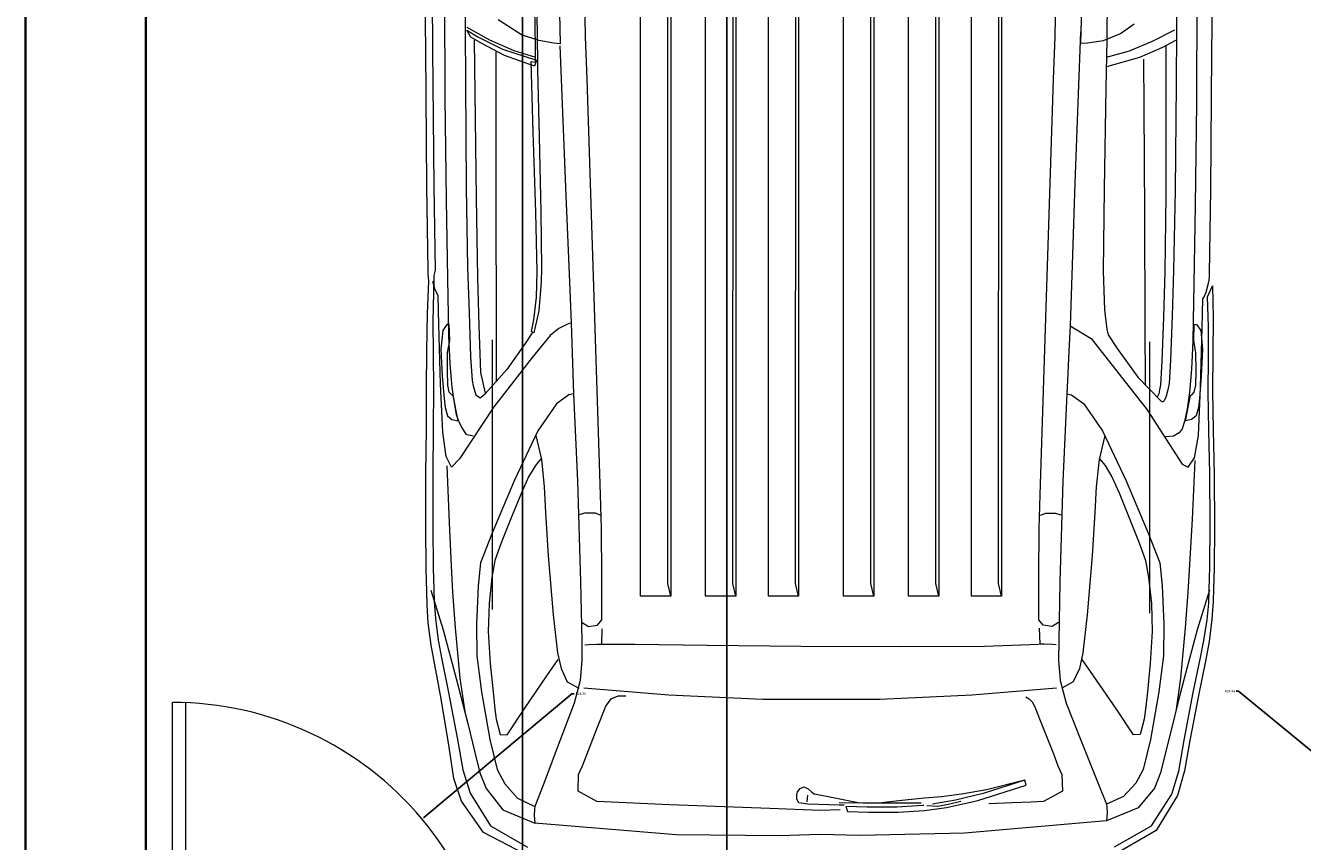
# Model space of a CAD drawing. Units: inches. Extents: x 5 to 421, y -617 to 43.
# Tile 2 of 15: x 37 to 133, y -566 to -505. Entities that reach past the tile are written whole.
import ezdxf

# ---------------------------------------------------------------- set-up
doc = ezdxf.new("R2010")
doc.units = ezdxf.units.IN
doc.header["$MEASUREMENT"] = 0
for name, color, linetype, lineweight in [('A-ANNO-DIMS', 2, 'Continuous', 18), ('A-SITE-GATE', 3, 'Continuous', 20), ('A-SITE-VEHC', 8, 'Continuous', 13), ('A-WALL', 7, 'Continuous', 35)]:
    doc.layers.add(name, color=color, linetype=linetype, lineweight=lineweight)
doc.styles.get("Standard").update_dxf_attribs({"font": 'arial.ttf'})
doc.dimstyles.get("Standard").update_dxf_attribs({"dimtxt": 0.18, "dimasz": 0.18, "dimexe": 0.18, "dimexo": 0.0625, "dimgap": 0.09, "dimtad": 0, "dimtih": 1, "dimtoh": 1, "dimdec": 0, "dimzin": 0, "dimdsep": 46, "dimlunit": 3, "dimtxsty": 'Standard', "dimcen": 0.09, "dimadec": 0, "dimazin": 0, "dimtfac": 1, "dimtdec": 0, "dimtofl": 0, "dimtmove": 0, "dimatfit": 3, "dimfxl": 1, "dimtolj": 1, "dimtzin": 0, "dimarcsym": 0})

# ---------------------------------------------------------------- blocks, each defined once
blk = doc.blocks.new('*D78')
at = {"layer": 'A-ANNO-DIMS', "color": 0, "lineweight": -2, "transparency": 16777216}
for p, q in [((74.624, -338.19), (74.624, -616.599)), ((89.924, -338.331), (89.924, -616.599)), ((74.804, -616.419), (81.958, -616.419)), ((89.744, -616.419), (82.589, -616.419))]:
    blk.add_line(p, q, dxfattribs=at)
at = {"layer": 'A-ANNO-DIMS', "color": 0, "transparency": 16777216}
for points in [[(74.804, -616.389), (74.804, -616.449), (74.624, -616.419)], [(89.744, -616.389), (89.744, -616.449), (89.924, -616.419)]]:
    blk.add_solid(points, dxfattribs=at)
at = {"layer": 'Defpoints', "color": 0, "transparency": 16777216}
for p in [(74.624, -338.127), (89.924, -338.269), (89.924, -616.419)]:
    blk.add_point(p, dxfattribs=at)
at = {"layer": 'A-ANNO-DIMS', "color": 0, "transparency": 16777216, "insert": (82.274, -616.419), "char_height": 0.18, "attachment_point": 5}
blk.add_mtext('\\A1;15.3', dxfattribs=at)
blk = doc.blocks.new('*D81')
at = {"layer": 'A-ANNO-DIMS', "color": 0, "lineweight": -2, "transparency": 16777216}
for p, q in [((78.334, -555.287), (67.254, -564.56)), ((78.514, -555.287), (78.334, -555.287)), ((48.33, -580.324), (48.51, -580.324)), ((48.42, -580.414), (48.42, -580.234))]:
    blk.add_line(p, q, dxfattribs=at)
at = {"layer": 'A-ANNO-DIMS', "color": 0, "transparency": 16777216}
blk.add_solid([(67.235, -564.537), (67.274, -564.583), (67.116, -564.676)], dxfattribs=at)
at = {"layer": 'Defpoints', "color": 0, "transparency": 16777216}
for p in [(67.116, -564.676), (48.42, -580.324)]:
    blk.add_point(p, dxfattribs=at)
at = {"layer": 'A-ANNO-DIMS', "color": 0, "transparency": 16777216, "insert": (78.994, -555.287), "char_height": 0.18, "attachment_point": 5}
blk.add_mtext('\\A1;R24.38', dxfattribs=at)
blk = doc.blocks.new('*D82')
at = {"layer": 'A-ANNO-DIMS', "color": 0, "lineweight": -2, "transparency": 16777216}
for p, q in [((128.083, -555.094), (128.263, -555.094)), ((128.263, -555.094), (139.433, -564.316)), ((158.33, -579.992), (158.51, -579.992)), ((158.42, -580.082), (158.42, -579.902))]:
    blk.add_line(p, q, dxfattribs=at)
at = {"layer": 'A-ANNO-DIMS', "color": 0, "transparency": 16777216}
blk.add_solid([(139.452, -564.293), (139.414, -564.339), (139.572, -564.431)], dxfattribs=at)
at = {"layer": 'Defpoints', "color": 0, "transparency": 16777216}
for p in [(139.572, -564.431), (158.42, -579.992)]:
    blk.add_point(p, dxfattribs=at)
at = {"layer": 'A-ANNO-DIMS', "color": 0, "transparency": 16777216, "insert": (127.603, -555.094), "char_height": 0.18, "attachment_point": 5}
blk.add_mtext('\\A1;R24.44', dxfattribs=at)

msp = doc.modelspace()

# ---------------------------------------------------------------- linework, layer by layer
at = {"layer": 'A-SITE-GATE'}
for p, q in [((48.4196, -579.9431), (48.4196, -555.9431)), ((49.4196, -579.9431), (49.4196, -555.9431))]:
    msp.add_line(p, q, dxfattribs=at)
msp.add_arc((48.4196, -580.3243), 24.3812, 349.855002, 90, dxfattribs=at)
at = {"layer": 'A-SITE-VEHC'}
for p, q in [((83.4744, -547.9801), (83.4744, -488.6203)), ((85.7354, -488.6203), (85.7354, -547.9801)), ((85.7372, -488.6203), (85.7372, -547.9801)), ((88.3484, -547.9801), (88.3484, -488.6203)), ((90.6093, -488.6203), (90.6093, -547.9801)), ((90.6116, -488.6203), (90.6116, -547.9801)), ((93.0486, -547.9801), (93.0486, -488.6203)), ((95.3095, -488.6203), (95.3095, -547.9801)), ((95.3114, -488.6203), (95.3114, -547.9801)), ((98.6716, -547.9801), (98.6716, -488.6203)), ((100.9326, -488.6203), (100.9326, -547.9801)), ((100.9348, -488.6203), (100.9348, -547.9801)), ((103.5459, -547.9801), (103.5459, -488.6203)), ((105.8069, -488.6203), (105.8069, -547.9801)), ((105.8088, -488.6203), (105.8088, -547.9801)), ((108.2458, -547.9801), (108.2458, -488.6203)), ((110.509, -488.6203), (110.509, -547.9801)), ((85.5102, -547.0362), (85.5319, -488.8077)), ((90.3843, -547.0362), (90.4059, -488.8077)), ((95.0844, -547.0362), (95.106, -488.8077)), ((100.7075, -547.0362), (100.7295, -488.8077)), ((105.5818, -547.0362), (105.6034, -488.8077)), ((110.2835, -547.0362), (110.3055, -488.8077)), ((77.319, -500.0842), (77.4499, -506.6078)), ((70.3187, -500.3131), (70.3404, -505.5354)), ((116.593, -500.3246), (116.4284, -506.5623)), ((118.4468, -500.3246), (118.3945, -506.2816)), ((123.5984, -500.6219), (123.6155, -505.6028)), ((67.3848, -507.06), (67.339, -501.7004)), ((67.8614, -501.7001), (67.907, -507.0546)), ((126.2663, -507.3072), (126.312, -501.9535)), ((68.7799, -502.4435), (68.8237, -510.6554)), ((125.1395, -502.8364), (125.0956, -511.048)), ((79.3514, -506.1001), (79.2954, -503.1925)), ((114.5196, -506.1001), (114.5618, -503.1925)), ((74.5618, -505.9489), (72.8057, -504.82)), ((75.5955, -507.9943), (75.5741, -504.1995)), ((75.6999, -503.9859), (75.7273, -506.4716)), ((70.3404, -505.5354), (70.3623, -509.4903)), ((70.4624, -505.3758), (72.1516, -506.323)), ((70.7756, -506.123), (70.4709, -505.6006)), ((70.4709, -505.6006), (71.2991, -506.0794)), ((116.4246, -505.7177), (116.0042, -517.0399)), ((118.1321, -506.3538), (119.4056, -505.8321)), ((119.4056, -505.8321), (120.4408, -505.1144)), ((123.4596, -505.5857), (121.8455, -506.4111)), ((123.6155, -505.6028), (123.5823, -509.6026)), ((71.5768, -506.5812), (70.7756, -506.123)), ((71.015, -506.3404), (71.0577, -510.2878)), ((71.2991, -506.0794), (73.1357, -507.0166)), ((73.2844, -507.4853), (71.5768, -506.5812)), ((72.1516, -506.323), (73.9774, -507.1267)), ((75.8522, -506.3712), (74.5618, -505.9489)), ((75.7273, -506.4716), (75.7321, -506.7248)), ((75.7321, -506.7248), (75.7455, -507.4366)), ((76.9719, -506.5627), (75.8522, -506.3712)), ((77.4499, -506.6078), (76.9719, -506.5627)), ((77.4324, -506.7565), (77.8753, -517.9769)), ((79.4666, -509.273), (79.3514, -506.1001)), ((114.4044, -509.273), (114.5196, -506.1001)), ((116.4284, -506.5623), (116.9495, -506.5392)), ((116.9495, -506.5392), (118.1321, -506.3538)), ((118.3945, -506.2816), (118.3208, -509.9451)), ((121.8455, -506.4111), (120.0535, -507.1731)), ((122.5855, -506.8683), (123.5592, -506.3357)), ((67.4807, -517.2812), (67.3848, -507.06)), ((67.907, -507.0546), (68.0026, -517.266)), ((72.6253, -507.2108), (72.6407, -518.9773)), ((73.1357, -507.0166), (75.6824, -507.8316)), ((75.5312, -508.2977), (73.2844, -507.4853)), ((73.9774, -507.1267), (75.6063, -507.6244)), ((75.7455, -507.4366), (75.7661, -508.5345)), ((120.0535, -507.1731), (118.3383, -507.6298)), ((118.3945, -508.3041), (120.8525, -507.6176)), ((120.8525, -507.6176), (122.5855, -506.8683)), ((122.8025, -506.7973), (122.8107, -510.5099)), ((126.1706, -517.5172), (126.2663, -507.3072)), ((75.4444, -513.2208), (75.2799, -507.9507)), ((75.2799, -507.9507), (75.5955, -507.9943)), ((75.6824, -507.8316), (75.5312, -508.2977)), ((75.7661, -508.5345), (75.8774, -513.5869)), ((121.1489, -507.7549), (121.1657, -511.3489)), ((70.3623, -509.4903), (70.4245, -517.4023)), ((79.6696, -515.5089), (79.4666, -509.273)), ((114.2014, -515.5089), (114.4044, -509.273)), ((123.5823, -509.6026), (123.499, -517.5978)), ((71.0577, -510.2878), (71.1584, -518.1856)), ((118.3208, -509.9451), (118.1837, -517.4658)), ((122.8107, -510.5099), (122.8046, -517.972)), ((68.8237, -510.6554), (68.9202, -518.3353)), ((121.1657, -511.3489), (121.2025, -519.3695)), ((125.0956, -511.048), (124.9992, -518.7279)), ((75.6306, -519.2183), (75.4444, -513.2208)), ((75.8774, -513.5869), (76.0031, -519.1903)), ((79.9166, -523.2738), (79.6696, -515.5089)), ((113.9543, -523.2738), (114.2014, -515.5089)), ((67.564, -523.5774), (67.4807, -517.2812)), ((68.0026, -517.266), (68.0858, -523.5564)), ((116.0042, -517.0399), (115.7383, -524.6937)), ((70.4245, -517.4023), (70.5216, -523.3421)), ((71.1584, -518.1856), (71.2761, -524.118)), ((77.8753, -517.9769), (78.1682, -525.0429)), ((118.1837, -517.4658), (118.11, -523.6388)), ((122.8046, -517.972), (122.7379, -523.6697)), ((123.499, -517.5978), (123.3908, -523.5825)), ((126.0872, -523.8072), (126.1706, -517.5172)), ((68.9202, -518.3353), (69.0167, -524.1928)), ((72.6407, -518.9773), (72.6513, -527.3867)), ((75.7368, -523.6611), (75.6306, -519.2183)), ((76.0031, -519.1903), (76.0628, -523.4093)), ((124.9992, -518.7279), (124.9026, -524.5855)), ((121.2025, -519.3695), (121.2393, -527.6745)), ((67.5718, -523.843), (67.564, -523.5774)), ((67.5842, -524.1086), (67.5718, -523.843)), ((67.9959, -523.967), (67.9903, -524.1832)), ((68.0548, -523.7749), (67.9959, -523.967)), ((68.0858, -523.5564), (68.0548, -523.7749)), ((70.5216, -523.3421), (70.6337, -526.7524)), ((75.6704, -525.6251), (75.7368, -523.6611)), ((76.0628, -523.4093), (76.0244, -524.4781)), ((80.1637, -531.0339), (79.9166, -523.2738)), ((113.7073, -531.0339), (113.9543, -523.2738)), ((118.11, -523.6388), (118.2119, -526.5496)), ((122.7379, -523.6697), (122.6256, -527.0799)), ((123.3908, -523.5825), (123.2784, -526.9928)), ((126.0712, -524.0753), (126.0872, -523.8072)), ((67.5231, -526.8298), (67.6166, -524.3723)), ((67.6166, -524.3723), (67.5842, -524.1086)), ((68.0933, -525.0349), (67.921, -524.4245)), ((67.9903, -524.1832), (67.9687, -525.206)), ((69.0167, -524.1928), (69.0606, -526.9376)), ((71.2761, -524.118), (71.3615, -527.7011)), ((76.0244, -524.4781), (75.8557, -526.6231)), ((115.7383, -524.6937), (115.6386, -527.7255)), ((124.9026, -524.5855), (124.8587, -527.3304)), ((125.8378, -525.2254), (126.0137, -524.543)), ((125.936, -525.576), (126.2938, -524.7368)), ((126.0137, -524.543), (126.0462, -524.3203)), ((126.0462, -524.3203), (126.0712, -524.0753)), ((126.2938, -524.7368), (126.3474, -527.1415)), ((67.9687, -525.206), (67.9191, -527.4442)), ((68.2573, -525.3729), (68.0933, -525.0349)), ((68.3304, -525.477), (68.2573, -525.3729)), ((68.3803, -527.641), (68.3304, -525.477)), ((75.4929, -527.2988), (75.6704, -525.6251)), ((78.1682, -525.0429), (78.2741, -527.4995)), ((125.5318, -527.8813), (125.5817, -525.7173)), ((125.5817, -525.7173), (125.6618, -525.6019)), ((125.6618, -525.6019), (125.8378, -525.2254)), ((125.9974, -527.7842), (125.936, -525.576)), ((67.4669, -529.6087), (67.5231, -526.8298)), ((70.6337, -526.7524), (70.746, -530.0629)), ((75.8557, -526.6231), (75.4761, -528.2518)), ((118.2119, -526.5496), (118.4012, -528.0123)), ((67.9191, -527.4442), (67.9451, -529.822)), ((68.5052, -532.077), (68.3803, -527.641)), ((68.9784, -527.6272), (68.6616, -528.0736)), ((69.1545, -527.5995), (68.9784, -527.6272)), ((69.0606, -526.9376), (69.096, -528.4983)), ((69.186, -528.8601), (69.1545, -527.5995)), ((71.3615, -527.7011), (71.4977, -531.2238)), ((72.6513, -527.3867), (72.6561, -531.8813)), ((75.3016, -528.1645), (75.4929, -527.2988)), ((77.9421, -527.6384), (77.3442, -527.9386)), ((78.2057, -527.5412), (77.9421, -527.6384)), ((78.2741, -527.4995), (78.4473, -532.8319)), ((115.6386, -527.7255), (115.5537, -529.6271)), ((115.6386, -527.7255), (117.211, -528.6949)), ((121.2393, -527.6745), (121.2559, -532.1217)), ((122.6256, -527.0799), (122.5132, -530.3902)), ((123.2784, -526.9928), (123.166, -530.3033)), ((124.8587, -527.3304), (124.8234, -528.8909)), ((124.9034, -528.8601), (124.9351, -527.5995)), ((124.9351, -527.5995), (125.1112, -527.6272)), ((125.1112, -527.6272), (125.4279, -528.0736)), ((125.9934, -530.1069), (125.9974, -527.7842)), ((126.3474, -527.1415), (126.3281, -529.8223)), ((68.6616, -528.0736), (68.5214, -529.4835)), ((69.096, -528.4983), (69.1939, -530.5832)), ((75.4089, -528.1738), (74.8288, -529.0713)), ((75.4761, -528.2518), (75.3016, -528.1645)), ((76.7011, -528.4546), (75.359, -530.1128)), ((77.3442, -527.9386), (76.7011, -528.4546)), ((117.211, -528.6949), (121.4244, -534.0318)), ((118.4012, -528.0123), (118.5031, -528.4138)), ((118.5031, -528.4138), (119.1732, -529.4459)), ((125.407, -532.3174), (125.5318, -527.8813)), ((125.4279, -528.0736), (125.568, -529.4835)), ((67.4482, -532.4362), (67.4669, -529.6087)), ((68.5214, -529.4835), (68.6248, -531.5112)), ((69.0205, -531.1087), (69.0266, -529.7416)), ((69.0266, -529.7416), (69.186, -528.8601)), ((72.3626, -528.7958), (72.3626, -548.9893)), ((74.8288, -529.0713), (73.4568, -531.0012)), ((115.5537, -529.6271), (115.4555, -531.7969)), ((119.1732, -529.4459), (120.7171, -531.5766)), ((121.5864, -528.941), (121.5864, -549.244)), ((124.8234, -528.8909), (124.7256, -530.9758)), ((125.0629, -529.7416), (124.9034, -528.8601)), ((125.0691, -531.1087), (125.0629, -529.7416)), ((125.568, -529.4835), (125.4646, -531.5112)), ((67.9451, -529.822), (67.9706, -532.4362)), ((69.1939, -530.5832), (69.3417, -532.3309)), ((70.746, -530.0629), (70.8583, -531.8253)), ((75.359, -530.1128), (73.4552, -532.5451)), ((122.5132, -530.3902), (122.4008, -532.1526)), ((123.166, -530.3033), (123.0537, -532.0656)), ((125.9797, -532.6912), (125.9934, -530.1069)), ((126.3281, -529.8223), (126.306, -532.6043)), ((68.6248, -531.5112), (68.7626, -533.173)), ((69.0457, -532.1907), (69.0205, -531.1087)), ((71.4977, -531.2238), (71.8421, -532.7784)), ((73.4568, -531.0012), (71.8449, -532.8195)), ((80.3667, -537.2555), (80.1637, -531.0339)), ((113.5043, -537.2555), (113.7073, -531.0339)), ((120.7171, -531.5766), (122.4358, -533.3578)), ((124.7256, -530.9758), (124.578, -532.7237)), ((125.0441, -532.1907), (125.0691, -531.1087)), ((125.4646, -531.5112), (125.3268, -533.173)), ((67.4335, -535.419), (67.4482, -532.4362)), ((67.9706, -532.4362), (67.9559, -535.419)), ((68.6675, -535.7016), (68.5052, -532.077)), ((69.1471, -532.7073), (69.0457, -532.1907)), ((69.3417, -532.3309), (69.5101, -533.4982)), ((70.8583, -531.8253), (70.9324, -532.2219)), ((70.9324, -532.2219), (71.1439, -532.9055)), ((73.4552, -532.5451), (72.4877, -533.7915)), ((115.4555, -531.7969), (115.4084, -532.8319)), ((122.3435, -532.5184), (122.2869, -532.8366)), ((122.4008, -532.1526), (122.3435, -532.5184)), ((122.9637, -532.5223), (122.8465, -533.0098)), ((123.0537, -532.0656), (122.9637, -532.5223)), ((124.9424, -532.7073), (125.0441, -532.1907)), ((125.2446, -535.9419), (125.407, -532.3174)), ((126.306, -532.6043), (126.3469, -535.5434)), ((68.7626, -533.173), (68.8314, -533.8618)), ((69.3357, -532.9144), (69.1471, -532.7073)), ((69.4373, -532.9523), (69.3357, -532.9144)), ((69.8071, -534.8455), (69.4373, -532.9523)), ((69.5101, -533.4982), (69.6786, -534.3658)), ((71.1439, -532.9055), (71.4766, -533.1175)), ((71.4766, -533.1175), (71.5968, -533.0275)), ((71.5968, -533.0275), (71.7197, -532.9279)), ((71.7197, -532.9279), (71.8449, -532.8195)), ((78.1103, -532.8968), (77.1829, -533.5772)), ((78.4473, -532.8319), (78.1103, -532.8968)), ((78.4473, -532.8319), (78.7592, -539.3815)), ((115.4084, -532.8319), (115.0965, -539.3815)), ((115.4084, -532.8319), (115.7454, -532.8968)), ((115.7454, -532.8968), (116.6727, -533.5772)), ((122.2869, -532.8366), (122.1498, -533.0828)), ((122.4358, -533.3578), (122.5259, -533.3999)), ((122.5259, -533.3999), (122.6059, -533.3943)), ((122.6059, -533.3943), (122.6767, -533.347)), ((122.8465, -533.0098), (122.6767, -533.347)), ((124.2822, -534.8455), (124.6521, -532.9523)), ((124.578, -532.7237), (124.4017, -533.9435)), ((124.6521, -532.9523), (124.7538, -532.9144)), ((124.7538, -532.9144), (124.9424, -532.7073)), ((125.3268, -533.173), (125.2579, -533.8618)), ((126.0191, -535.5652), (125.9797, -532.6912)), ((68.8314, -533.8618), (69.0077, -534.468)), ((69.0077, -534.468), (69.3467, -534.76)), ((69.6786, -534.3658), (69.8472, -534.8588)), ((72.4877, -533.7915), (69.9272, -537.696)), ((77.1829, -533.5772), (75.7909, -535.6012)), ((116.6727, -533.5772), (118.0645, -535.6012)), ((121.4244, -534.0318), (124.0211, -538.0876)), ((124.4017, -533.9435), (124.219, -534.9089)), ((125.0817, -534.468), (124.7427, -534.76)), ((125.2579, -533.8618), (125.0817, -534.468)), ((67.4064, -538.854), (67.4335, -535.419)), ((67.9559, -535.419), (67.9286, -538.854)), ((69.3467, -534.76), (69.8071, -534.8455)), ((69.8472, -534.8588), (70.0572, -535.322)), ((70.0572, -535.322), (70.3951, -535.8462)), ((124.0428, -535.4548), (123.8011, -535.7561)), ((124.219, -534.9089), (124.0428, -535.4548)), ((124.7427, -534.76), (124.2822, -534.8455)), ((68.9093, -537.5164), (68.6675, -535.7016)), ((70.3951, -535.8462), (70.9281, -535.9769)), ((75.7909, -535.6012), (74.0119, -539.3333)), ((75.6216, -535.9403), (76.0506, -537.7488)), ((118.2341, -535.9403), (117.8051, -537.7488)), ((118.0645, -535.6012), (119.8437, -539.3333)), ((123.3961, -536.0007), (122.8025, -536.0422)), ((123.8011, -535.7561), (123.3961, -536.0007)), ((124.9444, -537.6291), (125.2446, -535.9419)), ((126.0924, -538.7978), (126.0191, -535.5652)), ((126.3469, -535.5434), (126.4229, -538.8975)), ((80.4819, -540.4049), (80.3667, -537.2555)), ((113.3891, -540.4049), (113.5043, -537.2555)), ((69.3188, -538.3137), (68.9093, -537.5164)), ((68.9696, -538.2182), (69.1452, -542.4963)), ((69.9272, -537.696), (69.3188, -538.3137)), ((75.5984, -538.201), (75.0793, -539.0487)), ((76.017, -537.6922), (75.5984, -538.201)), ((76.0506, -537.7488), (76.2661, -539.7834)), ((117.8051, -537.7488), (117.5895, -539.7834)), ((117.8384, -537.6922), (118.2572, -538.201)), ((118.2572, -538.201), (118.7763, -539.0487)), ((124.0211, -538.0876), (124.4847, -538.3324)), ((124.4847, -538.3324), (124.9444, -537.6291)), ((124.9785, -537.8265), (124.7789, -542.2063)), ((67.3918, -542.7785), (67.4064, -538.854)), ((67.9286, -538.854), (67.9139, -542.7785)), ((75.0793, -539.0487), (74.5477, -540.2356)), ((118.7763, -539.0487), (119.308, -540.2356)), ((126.1318, -542.6136), (126.0924, -538.7978)), ((126.4229, -538.8975), (126.4639, -542.7785)), ((74.0119, -539.3333), (72.3332, -543.3041)), ((74.5477, -540.2356), (73.8465, -541.9938)), ((76.2661, -539.7834), (76.3561, -541.7051)), ((78.7592, -539.3815), (78.9832, -546.9106)), ((115.0965, -539.3815), (114.8725, -546.9106)), ((117.5895, -539.7834), (117.4994, -541.7051)), ((119.308, -540.2356), (120.0092, -541.9938)), ((119.8437, -539.3333), (121.5225, -543.3041)), ((80.5451, -542.9415), (80.4819, -540.4049)), ((113.3259, -542.9415), (113.3891, -540.4049)), ((73.8465, -541.9938), (73.0448, -543.9781)), ((76.3561, -541.7051), (76.5655, -544.9577)), ((78.892, -541.8738), (79.3034, -541.742)), ((79.3034, -541.742), (80.0653, -541.7481)), ((80.0653, -541.7481), (80.4695, -541.9063)), ((113.8056, -541.7916), (113.4015, -541.9498)), ((114.5676, -541.7855), (113.8056, -541.7916)), ((114.9789, -541.9174), (114.5676, -541.7855)), ((117.4994, -541.7051), (117.2901, -544.9577)), ((120.0092, -541.9938), (120.8109, -543.9781)), ((67.4173, -545.9493), (67.3918, -542.7785)), ((67.9139, -542.7785), (67.9432, -545.8744)), ((69.1452, -542.4963), (69.3045, -545.7157)), ((80.5743, -546.4804), (80.5451, -542.9415)), ((113.2968, -546.4804), (113.3259, -542.9415)), ((124.7789, -542.2063), (124.5751, -545.6142)), ((126.1036, -545.7877), (126.1318, -542.6136)), ((126.4639, -542.7785), (126.4345, -545.8744)), ((72.3332, -543.3041), (71.496, -545.4916)), ((73.0448, -543.9781), (72.5699, -545.3219)), ((120.8109, -543.9781), (121.2858, -545.3219)), ((121.5225, -543.3041), (122.3597, -545.4916)), ((76.5655, -544.9577), (76.9381, -549.3784)), ((117.2901, -544.9577), (116.9176, -549.3784)), ((67.4644, -547.6395), (67.4173, -545.9493)), ((67.9432, -545.8744), (67.9976, -547.4254)), ((69.3045, -545.7157), (69.4048, -547.6955)), ((71.496, -545.4916), (71.3222, -547.2182)), ((72.5699, -545.3219), (72.3499, -546.5861)), ((121.2858, -545.3219), (121.5058, -546.5861)), ((122.3597, -545.4916), (122.5335, -547.2182)), ((124.5751, -545.6142), (124.4509, -547.6955)), ((126.0512, -547.484), (126.1036, -545.7877)), ((126.4345, -545.8744), (126.3801, -547.4254)), ((72.3499, -546.5861), (72.1301, -548.5411)), ((78.9832, -546.9106), (79.069, -551.3127)), ((80.5758, -549.7451), (80.5743, -546.4804)), ((113.2955, -549.7451), (113.2968, -546.4804)), ((114.8725, -546.9106), (114.7867, -551.3127)), ((121.5058, -546.5861), (121.7256, -548.5411)), ((67.4899, -548.6627), (67.4644, -547.6395)), ((67.7659, -547.5258), (68.6973, -550.4961)), ((67.9976, -547.4254), (68.027, -548.3736)), ((69.4048, -547.6955), (69.589, -550.3497)), ((71.3222, -547.2182), (71.1987, -550.0754)), ((85.7354, -547.9801), (85.5102, -547.0362)), ((90.6093, -547.9801), (90.3843, -547.0362)), ((95.3095, -547.9801), (95.0844, -547.0362)), ((100.9326, -547.9801), (100.7075, -547.0362)), ((105.8069, -547.9801), (105.5818, -547.0362)), ((110.509, -547.9801), (110.2835, -547.0362)), ((122.5335, -547.2182), (122.657, -550.0754)), ((124.4509, -547.6955), (124.2666, -550.3497)), ((126.0898, -547.5258), (125.1583, -550.4961)), ((126.023, -548.5105), (126.0512, -547.484)), ((126.3801, -547.4254), (126.3509, -548.3736)), ((67.5746, -549.9914), (67.4899, -548.6627)), ((68.027, -548.3736), (68.1097, -549.6573)), ((72.1301, -548.5411), (72.0611, -550.6342)), ((85.7372, -547.9801), (83.4744, -547.9801)), ((90.6116, -547.9801), (88.3484, -547.9801)), ((95.3114, -547.9801), (93.0486, -547.9801)), ((100.9348, -547.9801), (98.6716, -547.9801)), ((105.8088, -547.9801), (103.5459, -547.9801)), ((110.509, -547.9801), (108.2458, -547.9801)), ((121.7256, -548.5411), (121.7946, -550.6342)), ((125.9157, -549.7556), (126.023, -548.5105)), ((126.3509, -548.3736), (126.2661, -549.7024)), ((68.1097, -549.6573), (68.3165, -551.2823)), ((76.9381, -549.3784), (77.2605, -552.2168)), ((80.2411, -550.1612), (80.5758, -549.7451)), ((113.6301, -550.1612), (113.2955, -549.7451)), ((116.9176, -549.3784), (116.5952, -552.2168)), ((125.6634, -551.3093), (125.9157, -549.7556)), ((126.2661, -549.7024), (126.0543, -551.3677)), ((67.7866, -551.6569), (67.5746, -549.9914)), ((68.6973, -550.4961), (69.6791, -554.1445)), ((69.589, -550.3497), (69.9364, -554.1216)), ((71.1987, -550.0754), (71.2133, -552.4428)), ((72.0611, -550.6342), (72.218, -553.0227)), ((79.0913, -549.9619), (79.5765, -550.2551)), ((79.5765, -550.2551), (80.2411, -550.1612)), ((80.5758, -550.4359), (80.5385, -551.595)), ((113.329, -550.3879), (113.3665, -551.5469)), ((114.2945, -550.2551), (113.6301, -550.1612)), ((114.78, -549.9619), (114.2945, -550.2551)), ((121.7946, -550.6342), (121.6375, -553.0227)), ((122.657, -550.0754), (122.6424, -552.4428)), ((124.2666, -550.3497), (123.9191, -554.1216)), ((125.1583, -550.4961), (124.1766, -554.1445)), ((68.0623, -553.1314), (67.7866, -551.6569)), ((68.3165, -551.2823), (68.585, -552.7214)), ((79.069, -551.3127), (79.0732, -552.7798)), ((79.5922, -551.637), (79.2951, -551.6517)), ((80.2035, -551.6098), (79.5922, -551.637)), ((80.5385, -551.595), (80.2035, -551.6098)), ((83.047, -551.6068), (80.5385, -551.595)), ((88.4652, -551.6704), (83.047, -551.6068)), ((95.4973, -551.7434), (88.4652, -551.6704)), ((113.3172, -551.595), (109.2192, -551.7481)), ((113.3665, -551.5469), (113.7014, -551.5616)), ((113.7014, -551.5616), (114.3126, -551.5889)), ((114.3126, -551.5889), (114.6096, -551.6036)), ((114.7867, -551.3127), (114.7825, -552.7798)), ((125.3703, -552.7099), (125.6634, -551.3093)), ((126.0543, -551.3677), (125.7788, -552.8423)), ((71.2133, -552.4428), (71.5712, -555.1577)), ((77.2605, -552.2168), (77.52, -553.3953)), ((102.8473, -551.7834), (95.4973, -551.7434)), ((109.2192, -551.7481), (102.8473, -551.7834)), ((116.5952, -552.2168), (116.3357, -553.3953)), ((122.6424, -552.4428), (122.2844, -555.1577)), ((68.5355, -555.6652), (68.0623, -553.1314)), ((68.585, -552.7214), (69.0975, -555.1956)), ((72.218, -553.0227), (72.4504, -555.3858)), ((76.4587, -553.9521), (77.3168, -552.7255)), ((77.52, -553.3953), (77.9805, -554.4105)), ((79.0732, -552.7798), (78.9518, -554.3099)), ((114.7825, -552.7798), (114.9039, -554.3099)), ((116.3357, -553.3953), (115.8752, -554.4105)), ((117.3968, -553.9521), (116.5386, -552.7255)), ((121.6375, -553.0227), (121.4052, -555.3858)), ((124.8576, -555.2096), (125.3703, -552.7099)), ((125.7788, -552.8423), (125.2697, -555.2998)), ((69.6791, -554.1445), (70.1962, -556.1729)), ((69.9364, -554.1216), (70.3089, -556.625)), ((74.7466, -556.4345), (76.4587, -553.9521)), ((77.9805, -554.4105), (78.843, -554.8731)), ((78.9518, -554.3099), (78.504, -556.0033)), ((114.9039, -554.3099), (115.3517, -556.0033)), ((115.8752, -554.4105), (115.0127, -554.8731)), ((119.109, -556.4345), (117.3968, -553.9521)), ((123.9191, -554.1216), (123.5465, -556.625)), ((124.1766, -554.1445), (123.6595, -556.1729)), ((69.0975, -555.1956), (69.7737, -558.7156)), ((71.5712, -555.1577), (72.1929, -558.7139)), ((72.4504, -555.3858), (72.5699, -556.4553)), ((85.5996, -555.4067), (79.2384, -554.8731)), ((81.2844, -555.6638), (81.8006, -555.442)), ((81.8006, -555.442), (82.3726, -555.4357)), ((92.6389, -555.7144), (85.5996, -555.4067)), ((108.3146, -555.4067), (101.3841, -555.7144)), ((114.617, -554.8731), (108.3146, -555.4067)), ((112.322, -555.5175), (112.5703, -555.6632)), ((121.4052, -555.3858), (121.2858, -556.4553)), ((122.2844, -555.1577), (121.6627, -558.7139)), ((124.1809, -558.7769), (124.8576, -555.2096)), ((125.2697, -555.2998), (124.5978, -558.796)), ((69.1407, -559.3036), (68.5355, -555.6652)), ((70.1962, -556.1729), (70.5308, -557.5271)), ((72.5699, -556.4553), (72.6661, -557.1921)), ((73.474, -558.3769), (74.7466, -556.4345)), ((78.504, -556.0033), (77.4405, -558.8126)), ((80.1972, -557.9143), (80.8776, -556.2293)), ((80.8776, -556.2293), (81.2844, -555.6638)), ((97.0407, -555.7206), (92.6389, -555.7144)), ((101.3841, -555.7144), (97.0407, -555.7206)), ((112.5703, -555.6632), (112.7913, -555.8951)), ((112.7913, -555.8951), (112.9781, -556.2293)), ((112.9781, -556.2293), (113.6585, -557.9143)), ((115.3517, -556.0033), (116.434, -558.7675)), ((120.3817, -558.3769), (119.109, -556.4345)), ((121.2858, -556.4553), (121.1896, -557.1921)), ((123.6595, -556.1729), (123.3246, -557.5271)), ((72.6661, -557.1921), (72.9633, -558.356)), ((121.1896, -557.1921), (120.8924, -558.356)), ((70.5308, -557.5271), (71.0667, -559.6977)), ((72.9633, -558.356), (73.474, -558.3769)), ((79.4666, -559.8004), (80.1972, -557.9143)), ((113.6585, -557.9143), (114.3891, -559.8004)), ((120.8924, -558.356), (120.3817, -558.3769)), ((123.3246, -557.5271), (122.7888, -559.6977)), ((69.5012, -561.6496), (69.1407, -559.3036)), ((69.7737, -558.7156), (70.1726, -561.0008)), ((72.1929, -558.7139), (72.7392, -560.9766)), ((77.4405, -558.8126), (76.1761, -562.1353)), ((116.434, -558.7675), (117.7335, -562.0063)), ((121.6627, -558.7139), (121.1165, -560.9766)), ((123.7817, -561.0874), (124.1809, -558.7769)), ((124.5978, -558.796), (124.2013, -561.0657)), ((71.0667, -559.6977), (71.4393, -561.2026)), ((79.1254, -560.6942), (79.4666, -559.8004)), ((114.3891, -559.8004), (114.7303, -560.6942)), ((122.7888, -559.6977), (122.4164, -561.2026)), ((70.1726, -561.0008), (70.7045, -562.7462)), ((71.4393, -561.2026), (71.9025, -562.3958)), ((72.7392, -560.9766), (73.3211, -562.0445)), ((78.8386, -561.3452), (79.1254, -560.6942)), ((114.7303, -560.6942), (115.017, -561.3452)), ((121.1165, -560.9766), (120.5535, -561.9994)), ((122.4164, -561.2026), (121.9721, -562.3507)), ((123.2599, -562.805), (123.7817, -561.0874)), ((124.2013, -561.0657), (123.6802, -562.909)), ((70.0619, -563.3417), (69.5012, -561.6496)), ((73.3211, -562.0445), (74.2673, -563.1233)), ((76.1761, -562.1353), (75.5649, -563.7389)), ((78.7904, -562.5863), (78.8386, -561.3452)), ((108.7331, -563.2908), (112.3589, -562.1367)), ((112.2446, -561.761), (109.1262, -562.7663)), ((112.2446, -561.761), (109.3763, -562.4808)), ((112.3589, -562.1367), (112.2446, -561.761)), ((115.017, -561.3452), (115.0651, -562.5863)), ((117.7335, -562.0063), (118.3637, -563.5648)), ((120.5535, -561.9994), (119.6426, -562.9943)), ((70.7045, -562.7462), (72.2382, -565.178)), ((71.9025, -562.3958), (73.1694, -563.9768)), ((74.2673, -563.1233), (75.5649, -563.7389)), ((80.1992, -563.3502), (78.7904, -562.5863)), ((95.1681, -562.8498), (95.2268, -562.6309)), ((95.1781, -563.1793), (95.1681, -562.8498)), ((95.3249, -563.4692), (95.1781, -563.1793)), ((95.2268, -562.6309), (95.4294, -562.3759)), ((95.4294, -562.3759), (95.7123, -562.2624)), ((95.7123, -562.2624), (96.0232, -562.405)), ((95.9611, -563.3907), (95.9968, -562.8794)), ((96.0232, -562.405), (96.3049, -562.6591)), ((96.3049, -562.6591), (96.5097, -562.8154)), ((96.7602, -562.8588), (96.5097, -562.8154)), ((97.7616, -563.0506), (96.7602, -562.8588)), ((99.8884, -563.4833), (97.7616, -563.0506)), ((104.7396, -563.1236), (103.0306, -563.2797)), ((106.0116, -563.0013), (104.7396, -563.1236)), ((107.5147, -562.8176), (106.0116, -563.0013)), ((109.1262, -562.7663), (107.0522, -563.2633)), ((109.3763, -562.4808), (107.5147, -562.8176)), ((115.0651, -562.5863), (113.6562, -563.3502)), ((119.6426, -562.9943), (118.3637, -563.5648)), ((121.9721, -562.3507), (120.7403, -563.8478)), ((121.7446, -565.1852), (123.2599, -562.805)), ((123.6802, -562.909), (122.0961, -565.5274)), ((71.7198, -565.6789), (70.0619, -563.3417)), ((73.1694, -563.9768), (75.5649, -564.9824)), ((75.5398, -563.9357), (75.5147, -564.4087)), ((75.5649, -563.7389), (75.5398, -563.9357)), ((85.6666, -563.6016), (80.1992, -563.3502)), ((93.1559, -563.8905), (85.6666, -563.6016)), ((96.9277, -564.0287), (93.1559, -563.8905)), ((96.0019, -563.5724), (95.3249, -563.4692)), ((98.3743, -563.631), (96.0019, -563.5724)), ((98.4319, -563.9738), (96.9277, -564.0287)), ((100.1221, -563.4798), (98.3517, -563.4709)), ((98.7098, -563.6342), (98.3743, -563.631)), ((100.4537, -563.7767), (98.8483, -563.7278)), ((98.8483, -563.7278), (98.9623, -564.1035)), ((98.9623, -564.1035), (100.5679, -564.1523)), ((102.9905, -563.4866), (100.1221, -563.4798)), ((102.6597, -563.7775), (100.4537, -563.7767)), ((100.5679, -564.1523), (102.7739, -564.1531)), ((103.0306, -563.2797), (101.3133, -563.4795)), ((104.6115, -563.6689), (102.6597, -563.7775)), ((102.7739, -564.1531), (104.7258, -564.0445)), ((104.494, -563.4893), (102.9905, -563.4866)), ((104.6335, -563.6661), (104.6115, -563.6689)), ((104.6556, -563.6634), (104.6335, -563.6661)), ((104.6783, -563.6606), (104.6556, -563.6634)), ((104.7258, -564.0445), (106.3946, -563.8183)), ((105.7267, -563.7406), (104.9008, -563.6785)), ((107.0522, -563.2633), (105.3399, -563.561)), ((105.9837, -563.6923), (105.7267, -563.7406)), ((106.6248, -563.5611), (105.9837, -563.6923)), ((106.3946, -563.8183), (108.7331, -563.2908)), ((107.4547, -563.3671), (106.6248, -563.5611)), ((111.2953, -563.4701), (109.5469, -563.5457)), ((112.703, -563.4038), (111.2953, -563.4701)), ((113.6562, -563.3502), (112.703, -563.4038)), ((118.3637, -563.5648), (118.3888, -563.7616)), ((120.7403, -563.8478), (118.3637, -564.8083)), ((118.3888, -563.7616), (118.414, -564.2348)), ((75.5147, -564.4087), (75.5649, -564.9824)), ((86.1376, -565.857), (75.5649, -564.9824)), ((118.3637, -564.8083), (107.7429, -565.7281)), ((118.414, -564.2348), (118.3637, -564.8083)), ((74.7792, -567.2796), (71.7198, -565.6789)), ((72.2382, -565.178), (75.0189, -566.7885)), ((93.8718, -565.9419), (86.1376, -565.857)), ((96.8713, -565.8369), (93.8718, -565.9419)), ((99.9191, -565.8967), (96.8713, -565.8369)), ((107.7429, -565.7281), (99.9191, -565.8967)), ((118.974, -566.7678), (121.7446, -565.1852)), ((122.0961, -565.5274), (119.0765, -567.2796))]:
    msp.add_line(p, q, dxfattribs=at)
at = {"layer": 'A-WALL'}
for p, q in [((37.4196, 10.8812), (37.4196, -584.6188)), ((46.4196, -395.6188), (46.4196, -584.6188))]:
    msp.add_line(p, q, dxfattribs=at)

# ---------------------------------------------------------------- dimensions: what is measured, and where the dimension line sits
at = {"layer": 'A-ANNO-DIMS'}
dim = msp.add_linear_dim(base=(89.9238, -616.4188), p1=(74.6237, -338.1275), p2=(89.9238, -338.2687), dimstyle='Standard', override={"dimdec": 1, "dimlfac": 1, "dimrnd": 0, "dimzin": 0, "dimdsep": 46, "dimlunit": 2}, dxfattribs=at)
dim.commit()
dim.dimension.update_dxf_attribs({"geometry": '*D78', "text_midpoint": (82.2737, -616.4188)})
for center, mpoint, picture, middle in [((48.4196, -580.3243), (67.1163, -564.6758), '*D81', (78.9943, -555.2866)), ((158.4196, -579.9922), (139.5717, -564.4307), '*D82', (127.6034, -555.0938))]:
    dim = msp.add_radius_dim(center=center, mpoint=mpoint, dimstyle='Standard', override={"dimdec": 2, "dimlfac": 1, "dimrnd": 0, "dimzin": 0, "dimdsep": 46, "dimlunit": 2}, dxfattribs=at)
    dim.commit()
    dim.dimension.update_dxf_attribs({"geometry": picture, "text_midpoint": middle, "dimtype": 164})

doc.saveas('drawing.dxf')
